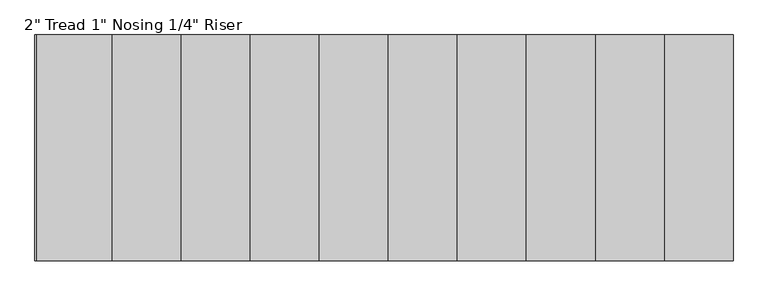
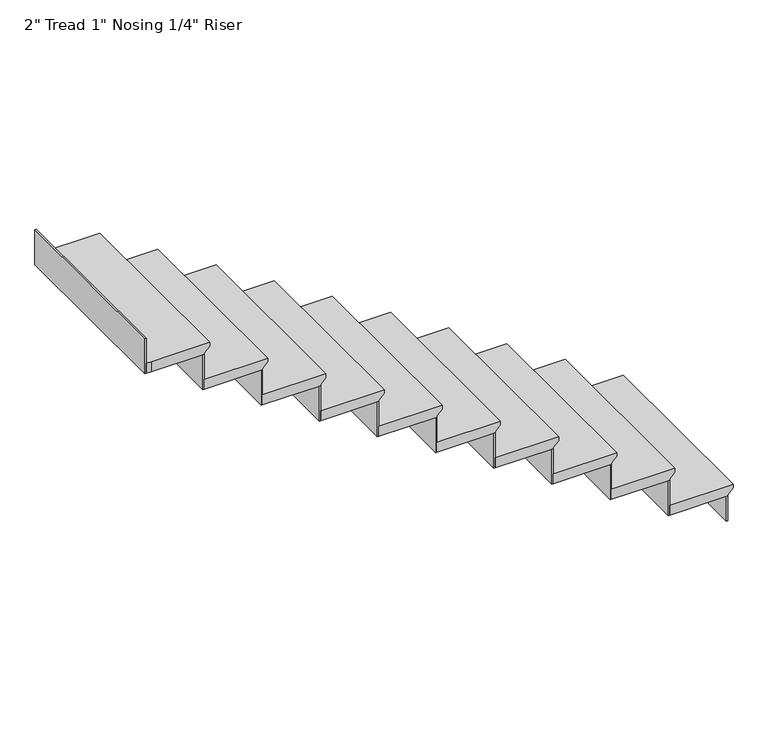
"""IFC4 building model written with IfcOpenShell, lengths in millimetres: stair flight geometry."""

from ifc_helpers import new_model, si_unit, origin, place, context, project, spatial, faceted_brep, source, transform, mapped, element, save


def stair_flight_440f75bd(model_context):
    return source(origin(), model_context, "Body", "Brep", [
        faceted_brep([(23001.1136801, 5080.9752787, 3968.75), (23001.1136801, 5080.9752787, 3987.8), (23001.1136801, 4166.5752787, 3987.8), (23001.1136801, 4166.5752787, 3968.75), (22975.7136801, 5080.9752787, 3943.35), (22975.7136801, 4166.5752787, 3943.35), (22696.3136801, 5080.9752787, 3987.8), (22696.3136801, 4166.5752787, 3987.8), (22975.7136801, 4166.5752787, 3937.0), (22696.3136801, 4166.5752787, 3937.0), (22696.3136801, 5080.9752787, 3937.0), (22975.7136801, 5080.9752787, 3937.0)], [[[0, 1, 2, 3]], [[4, 0, 3, 5]], [[2, 1, 6, 7]], [[8, 9, 10, 11]], [[2, 7, 9, 8, 5, 3]], [[8, 11, 4, 5]], [[6, 1, 0, 4, 11, 10]], [[7, 6, 10, 9]]]),
        faceted_brep([(22975.7136801, 5080.9752787, 3937.0), (22975.7136801, 5080.9752787, 3810.0), (22969.3636801, 5080.9752787, 3810.0), (22969.3636801, 5080.9752787, 3937.0), (22975.7136801, 4166.5752787, 3937.0), (22969.3636801, 4166.5752787, 3937.0), (22969.3636801, 4166.5752787, 3810.0), (22975.7136801, 4166.5752787, 3810.0)], [[[0, 1, 2, 3]], [[4, 5, 6, 7]], [[1, 0, 4, 7]], [[2, 1, 7, 6]], [[3, 2, 6, 5]], [[0, 3, 5, 4]]]),
        faceted_brep([(22696.3136801, 5080.9752787, 4114.8), (22696.3136801, 5080.9752787, 3937.0), (22689.9636801, 5080.9752787, 3937.0), (22689.9636801, 5080.9752787, 4114.8), (22696.3136801, 4166.5752787, 4114.8), (22689.9636801, 4166.5752787, 4114.8), (22689.9636801, 4166.5752787, 3937.0), (22696.3136801, 4166.5752787, 3937.0)], [[[0, 1, 2, 3]], [[4, 5, 6, 7]], [[1, 0, 4, 7]], [[2, 1, 7, 6]], [[3, 2, 6, 5]], [[0, 3, 5, 4]]]),
        faceted_brep([(22721.7136801, 4166.5752787, 4165.6), (22721.7136801, 5080.9752787, 4165.6), (22416.9136801, 5080.9752787, 4165.6), (22416.9136801, 4166.5752787, 4165.6), (22696.3136801, 4166.5752787, 4114.8), (22416.9136801, 4166.5752787, 4114.8), (22416.9136801, 5080.9752787, 4114.8), (22696.3136801, 5080.9752787, 4114.8), (22696.3136801, 4166.5752787, 4121.15), (22721.7136801, 4166.5752787, 4146.55), (22696.3136801, 5080.9752787, 4121.15), (22721.7136801, 5080.9752787, 4146.55)], [[[0, 1, 2, 3]], [[4, 5, 6, 7]], [[0, 3, 5, 4, 8, 9]], [[4, 7, 10, 8]], [[2, 1, 11, 10, 7, 6]], [[3, 2, 6, 5]], [[11, 1, 0, 9]], [[10, 11, 9, 8]]]),
        faceted_brep([(22416.9136801, 5080.9752787, 4292.6), (22416.9136801, 5080.9752787, 4114.8), (22410.5636801, 5080.9752787, 4114.8), (22410.5636801, 5080.9752787, 4292.6), (22416.9136801, 4166.5752787, 4292.6), (22410.5636801, 4166.5752787, 4292.6), (22410.5636801, 4166.5752787, 4114.8), (22416.9136801, 4166.5752787, 4114.8)], [[[0, 1, 2, 3]], [[4, 5, 6, 7]], [[1, 0, 4, 7]], [[2, 1, 7, 6]], [[3, 2, 6, 5]], [[0, 3, 5, 4]]]),
        faceted_brep([(22442.3136801, 4166.5752787, 4343.4), (22442.3136801, 5080.9752787, 4343.4), (22137.5136801, 5080.9752787, 4343.4), (22137.5136801, 4166.5752787, 4343.4), (22416.9136801, 4166.5752787, 4292.6), (22137.5136801, 4166.5752787, 4292.6), (22137.5136801, 5080.9752787, 4292.6), (22416.9136801, 5080.9752787, 4292.6), (22416.9136801, 4166.5752787, 4298.95), (22442.3136801, 4166.5752787, 4324.35), (22416.9136801, 5080.9752787, 4298.95), (22442.3136801, 5080.9752787, 4324.35)], [[[0, 1, 2, 3]], [[4, 5, 6, 7]], [[0, 3, 5, 4, 8, 9]], [[4, 7, 10, 8]], [[2, 1, 11, 10, 7, 6]], [[3, 2, 6, 5]], [[11, 1, 0, 9]], [[10, 11, 9, 8]]]),
        faceted_brep([(22137.5136801, 5080.9752787, 4470.4), (22137.5136801, 5080.9752787, 4292.6), (22131.1636801, 5080.9752787, 4292.6), (22131.1636801, 5080.9752787, 4470.4), (22137.5136801, 4166.5752787, 4470.4), (22131.1636801, 4166.5752787, 4470.4), (22131.1636801, 4166.5752787, 4292.6), (22137.5136801, 4166.5752787, 4292.6)], [[[0, 1, 2, 3]], [[4, 5, 6, 7]], [[1, 0, 4, 7]], [[2, 1, 7, 6]], [[3, 2, 6, 5]], [[0, 3, 5, 4]]]),
        faceted_brep([(22162.9136801, 4166.5752787, 4521.2), (22162.9136801, 5080.9752787, 4521.2), (21858.1136801, 5080.9752787, 4521.2), (21858.1136801, 4166.5752787, 4521.2), (22137.5136801, 4166.5752787, 4470.4), (21858.1136801, 4166.5752787, 4470.4), (21858.1136801, 5080.9752787, 4470.4), (22137.5136801, 5080.9752787, 4470.4), (22137.5136801, 4166.5752787, 4476.75), (22162.9136801, 4166.5752787, 4502.15), (22137.5136801, 5080.9752787, 4476.75), (22162.9136801, 5080.9752787, 4502.15)], [[[0, 1, 2, 3]], [[4, 5, 6, 7]], [[0, 3, 5, 4, 8, 9]], [[4, 7, 10, 8]], [[2, 1, 11, 10, 7, 6]], [[3, 2, 6, 5]], [[11, 1, 0, 9]], [[10, 11, 9, 8]]]),
        faceted_brep([(21858.1136801, 5080.9752787, 4648.2), (21858.1136801, 5080.9752787, 4470.4), (21851.7636801, 5080.9752787, 4470.4), (21851.7636801, 5080.9752787, 4648.2), (21858.1136801, 4166.5752787, 4648.2), (21851.7636801, 4166.5752787, 4648.2), (21851.7636801, 4166.5752787, 4470.4), (21858.1136801, 4166.5752787, 4470.4)], [[[0, 1, 2, 3]], [[4, 5, 6, 7]], [[1, 0, 4, 7]], [[2, 1, 7, 6]], [[3, 2, 6, 5]], [[0, 3, 5, 4]]]),
        faceted_brep([(21883.5136801, 4166.5752787, 4699.0), (21883.5136801, 5080.9752787, 4699.0), (21578.7136801, 5080.9752787, 4699.0), (21578.7136801, 4166.5752787, 4699.0), (21858.1136801, 4166.5752787, 4648.2), (21578.7136801, 4166.5752787, 4648.2), (21578.7136801, 5080.9752787, 4648.2), (21858.1136801, 5080.9752787, 4648.2), (21858.1136801, 4166.5752787, 4654.55), (21883.5136801, 4166.5752787, 4679.95), (21858.1136801, 5080.9752787, 4654.55), (21883.5136801, 5080.9752787, 4679.95)], [[[0, 1, 2, 3]], [[4, 5, 6, 7]], [[0, 3, 5, 4, 8, 9]], [[4, 7, 10, 8]], [[2, 1, 11, 10, 7, 6]], [[3, 2, 6, 5]], [[11, 1, 0, 9]], [[10, 11, 9, 8]]]),
        faceted_brep([(21578.7136801, 5080.9752787, 4826.0), (21578.7136801, 5080.9752787, 4648.2), (21572.3636801, 5080.9752787, 4648.2), (21572.3636801, 5080.9752787, 4826.0), (21578.7136801, 4166.5752787, 4826.0), (21572.3636801, 4166.5752787, 4826.0), (21572.3636801, 4166.5752787, 4648.2), (21578.7136801, 4166.5752787, 4648.2)], [[[0, 1, 2, 3]], [[4, 5, 6, 7]], [[1, 0, 4, 7]], [[2, 1, 7, 6]], [[3, 2, 6, 5]], [[0, 3, 5, 4]]]),
        faceted_brep([(21604.1136801, 4166.5752787, 4876.8), (21604.1136801, 5080.9752787, 4876.8), (21299.3136801, 5080.9752787, 4876.8), (21299.3136801, 4166.5752787, 4876.8), (21578.7136801, 4166.5752787, 4826.0), (21299.3136801, 4166.5752787, 4826.0), (21299.3136801, 5080.9752787, 4826.0), (21578.7136801, 5080.9752787, 4826.0), (21578.7136801, 4166.5752787, 4832.35), (21604.1136801, 4166.5752787, 4857.75), (21578.7136801, 5080.9752787, 4832.35), (21604.1136801, 5080.9752787, 4857.75)], [[[0, 1, 2, 3]], [[4, 5, 6, 7]], [[0, 3, 5, 4, 8, 9]], [[4, 7, 10, 8]], [[2, 1, 11, 10, 7, 6]], [[3, 2, 6, 5]], [[11, 1, 0, 9]], [[10, 11, 9, 8]]]),
        faceted_brep([(21299.3136801, 5080.9752787, 5003.8), (21299.3136801, 5080.9752787, 4826.0), (21292.9636801, 5080.9752787, 4826.0), (21292.9636801, 5080.9752787, 5003.8), (21299.3136801, 4166.5752787, 5003.8), (21292.9636801, 4166.5752787, 5003.8), (21292.9636801, 4166.5752787, 4826.0), (21299.3136801, 4166.5752787, 4826.0)], [[[0, 1, 2, 3]], [[4, 5, 6, 7]], [[1, 0, 4, 7]], [[2, 1, 7, 6]], [[3, 2, 6, 5]], [[0, 3, 5, 4]]]),
        faceted_brep([(21324.7136801, 4166.5752787, 5054.6), (21324.7136801, 5080.9752787, 5054.6), (21019.9136801, 5080.9752787, 5054.6), (21019.9136801, 4166.5752787, 5054.6), (21299.3136801, 4166.5752787, 5003.8), (21019.9136801, 4166.5752787, 5003.8), (21019.9136801, 5080.9752787, 5003.8), (21299.3136801, 5080.9752787, 5003.8), (21299.3136801, 4166.5752787, 5010.15), (21324.7136801, 4166.5752787, 5035.55), (21299.3136801, 5080.9752787, 5010.15), (21324.7136801, 5080.9752787, 5035.55)], [[[0, 1, 2, 3]], [[4, 5, 6, 7]], [[0, 3, 5, 4, 8, 9]], [[4, 7, 10, 8]], [[2, 1, 11, 10, 7, 6]], [[3, 2, 6, 5]], [[11, 1, 0, 9]], [[10, 11, 9, 8]]]),
        faceted_brep([(21019.9136801, 5080.9752787, 5181.6), (21019.9136801, 5080.9752787, 5003.8), (21013.5636801, 5080.9752787, 5003.8), (21013.5636801, 5080.9752787, 5181.6), (21019.9136801, 4166.5752787, 5181.6), (21013.5636801, 4166.5752787, 5181.6), (21013.5636801, 4166.5752787, 5003.8), (21019.9136801, 4166.5752787, 5003.8)], [[[0, 1, 2, 3]], [[4, 5, 6, 7]], [[1, 0, 4, 7]], [[2, 1, 7, 6]], [[3, 2, 6, 5]], [[0, 3, 5, 4]]]),
        faceted_brep([(21045.3136801, 4166.5752787, 5232.4), (21045.3136801, 5080.9752787, 5232.4), (20740.5136801, 5080.9752787, 5232.4), (20740.5136801, 4166.5752787, 5232.4), (21019.9136801, 4166.5752787, 5181.6), (20740.5136801, 4166.5752787, 5181.6), (20740.5136801, 5080.9752787, 5181.6), (21019.9136801, 5080.9752787, 5181.6), (21019.9136801, 4166.5752787, 5187.95), (21045.3136801, 4166.5752787, 5213.35), (21019.9136801, 5080.9752787, 5187.95), (21045.3136801, 5080.9752787, 5213.35)], [[[0, 1, 2, 3]], [[4, 5, 6, 7]], [[0, 3, 5, 4, 8, 9]], [[4, 7, 10, 8]], [[2, 1, 11, 10, 7, 6]], [[3, 2, 6, 5]], [[11, 1, 0, 9]], [[10, 11, 9, 8]]]),
        faceted_brep([(20740.5136801, 5080.9752787, 5359.4), (20740.5136801, 5080.9752787, 5181.6), (20734.1636801, 5080.9752787, 5181.6), (20734.1636801, 5080.9752787, 5359.4), (20740.5136801, 4166.5752787, 5359.4), (20734.1636801, 4166.5752787, 5359.4), (20734.1636801, 4166.5752787, 5181.6), (20740.5136801, 4166.5752787, 5181.6)], [[[0, 1, 2, 3]], [[4, 5, 6, 7]], [[1, 0, 4, 7]], [[2, 1, 7, 6]], [[3, 2, 6, 5]], [[0, 3, 5, 4]]]),
        faceted_brep([(20765.9136801, 4166.5752787, 5410.2), (20765.9136801, 5080.9752787, 5410.2), (20461.1136801, 5080.9752787, 5410.2), (20461.1136801, 4166.5752787, 5410.2), (20740.5136801, 4166.5752787, 5359.4), (20461.1136801, 4166.5752787, 5359.4), (20461.1136801, 5080.9752787, 5359.4), (20740.5136801, 5080.9752787, 5359.4), (20740.5136801, 4166.5752787, 5365.75), (20765.9136801, 4166.5752787, 5391.15), (20740.5136801, 5080.9752787, 5365.75), (20765.9136801, 5080.9752787, 5391.15)], [[[0, 1, 2, 3]], [[4, 5, 6, 7]], [[0, 3, 5, 4, 8, 9]], [[4, 7, 10, 8]], [[2, 1, 11, 10, 7, 6]], [[3, 2, 6, 5]], [[11, 1, 0, 9]], [[10, 11, 9, 8]]]),
        faceted_brep([(20181.7136801, 5080.9752787, 5715.0), (20181.7136801, 5080.9752787, 5537.2), (20175.3636801, 5080.9752787, 5537.2), (20175.3636801, 5080.9752787, 5715.0), (20181.7136801, 4166.5752787, 5715.0), (20175.3636801, 4166.5752787, 5715.0), (20175.3636801, 4166.5752787, 5537.2), (20181.7136801, 4166.5752787, 5537.2)], [[[0, 1, 2, 3]], [[4, 5, 6, 7]], [[1, 0, 4, 7]], [[2, 1, 7, 6]], [[3, 2, 6, 5]], [[0, 3, 5, 4]]]),
        faceted_brep([(20461.1136801, 5080.9752787, 5537.2), (20461.1136801, 5080.9752787, 5359.4), (20454.7636801, 5080.9752787, 5359.4), (20454.7636801, 5080.9752787, 5537.2), (20461.1136801, 4166.5752787, 5537.2), (20454.7636801, 4166.5752787, 5537.2), (20454.7636801, 4166.5752787, 5359.4), (20461.1136801, 4166.5752787, 5359.4)], [[[0, 1, 2, 3]], [[4, 5, 6, 7]], [[1, 0, 4, 7]], [[2, 1, 7, 6]], [[3, 2, 6, 5]], [[0, 3, 5, 4]]]),
        faceted_brep([(20181.7136801, 4166.5752787, 5588.0), (20207.1136801, 4166.5752787, 5588.0), (20486.5136801, 4166.5752787, 5588.0), (20486.5136801, 5080.9752787, 5588.0), (20181.7136801, 5080.9752787, 5588.0), (20207.1136801, 4166.5752787, 5537.2), (20181.7136801, 4166.5752787, 5537.2), (20181.7136801, 5080.9752787, 5537.2), (20461.1136801, 5080.9752787, 5537.2), (20461.1136801, 4166.5752787, 5537.2), (20461.1136801, 4166.5752787, 5543.55), (20486.5136801, 4166.5752787, 5568.95), (20461.1136801, 5080.9752787, 5543.55), (20486.5136801, 5080.9752787, 5568.95)], [[[0, 1, 2, 3, 4]], [[5, 6, 7, 8, 9]], [[1, 0, 6, 5]], [[2, 1, 5, 9, 10, 11]], [[9, 8, 12, 10]], [[4, 3, 13, 12, 8, 7]], [[0, 4, 7, 6]], [[13, 3, 2, 11]], [[12, 13, 11, 10]]]),
    ])


if __name__ == "__main__":
    model = new_model("IFC4")
    model_context = context("Model", 3, world=origin())
    ifc_project = project(units=[si_unit("LENGTHUNIT", "METRE", prefix="MILLI")], contexts=[model_context])
    site = spatial("IfcSite", under=ifc_project)
    building = spatial("IfcBuilding", under=site)
    placement = place(None, origin())
    stair_flight_shape = stair_flight_440f75bd(model_context)
    element("IfcStairFlight", 1, ObjectType="2\" Tread 1\" Nosing 1/4\" Riser", at=placement, inside=building, context=model_context, shape_type="MappedRepresentation", body=[
        mapped(stair_flight_shape, transform((0.0, 0.0, 0.0), x_axis=(1.0, 0.0, 0.0), y_axis=(0.0, 1.0, 0.0), z_axis=(0.0, 0.0, 1.0))),
    ])
    save(model, "model.ifc")
